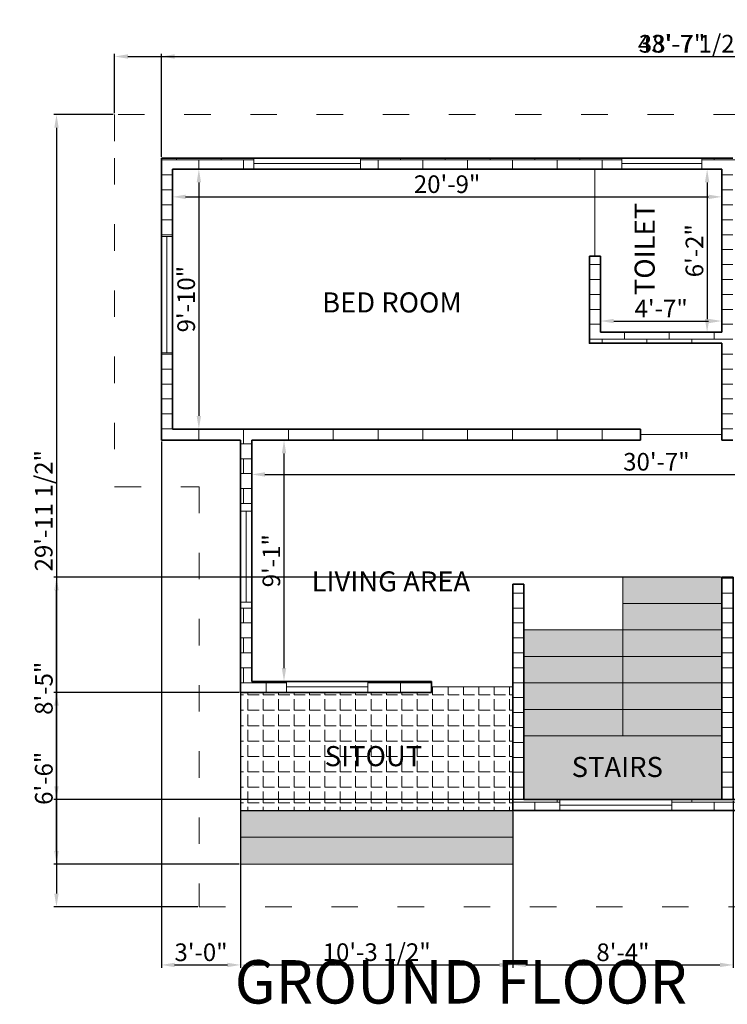
# Model space of a CAD drawing. Units: millimetres. Extents: x 1518 to 2850, y 936 to 2174.
# Tile 2 of 5: x 1686 to 2007, y 1697 to 2143. Entities that reach past the tile are written whole.
import ezdxf

# ---------------------------------------------------------------- set-up
doc = ezdxf.new("R2010")
doc.units = ezdxf.units.MM
doc.linetypes.add('ACAD_ISO03W100', pattern=[30, 12, -18])
for name, color, linetype, lineweight, true_color in [('A-ANNO-DIMS', 9, 'Continuous', 18, 0xafd9aa), ('A-ANNO-TEXT', 85, 'Continuous', 25, 0x58ba48), ('A-AREA-IDEN', 31, 'Continuous', 18, 0xfecc66), ('A-DOOR', 244, 'Continuous', 20, 0x991b1e), ('A-FLOR-PATT', 252, 'Continuous', 13, 0x939598), ('A-GLAZ', 141, 'Continuous', 18, 0xadddf7), ('A-ROOF-OVHD', 177, 'ACAD_ISO03W100', 18, 0x293189)]:
    doc.layers.add(name, color=color, linetype=linetype, lineweight=lineweight, true_color=true_color)
for name, color, linetype, lineweight in [('A-FLOR', 7, 'Continuous', 25), ('A-FLOR-STRS', 7, 'Continuous', 20), ('A-FLOR-STRS-PATT', 7, 'Continuous', 13), ('A-WALL', 7, 'Continuous', 35), ('A-WALL-PATT', 7, 'Continuous', 13)]:
    doc.layers.add(name, color=color, linetype=linetype, lineweight=lineweight)
doc.styles.get("Standard").update_dxf_attribs({"font": 'arial.ttf'})
doc.dimstyles.new('ISO-25', dxfattribs={"dimtxt": 8, "dimasz": 6, "dimexe": 1.25, "dimexo": 0.625, "dimtad": 1, "dimdec": 0, "dimlunit": 3, "dimtxsty": 'Standard', "dimcen": 2.5, "dimadec": 0, "dimazin": 0, "dimtfac": 1, "dimtdec": 0, "dimtmove": 0, "dimatfit": 3, "dimfxl": 1, "dimarcsym": 0})

# ---------------------------------------------------------------- blocks, each defined once
blk = doc.blocks.new('*D1')
at = {"layer": 'A-ANNO-DIMS', "color": 0, "lineweight": -2, "transparency": 16777216}
for p, q in [((1755, 2074.9), (1755, 2061.71)), ((2004.13, 2074.9), (2004.13, 2061.71)), ((1761, 2062.96), (1998.13, 2062.96))]:
    blk.add_line(p, q, dxfattribs=at)
at = {"layer": 'A-ANNO-DIMS', "color": 0, "transparency": 16777216}
for points in [[(1761, 2063.96), (1761, 2061.96), (1755, 2062.96)], [(1998.13, 2063.96), (1998.13, 2061.96), (2004.13, 2062.96)]]:
    blk.add_solid(points, dxfattribs=at)
at = {"layer": 'Defpoints', "color": 0, "transparency": 16777216}
for p in [(1755, 2075.52), (2004.13, 2075.52), (2004.13, 2062.96)]:
    blk.add_point(p, dxfattribs=at)
at = {"layer": 'A-ANNO-DIMS', "color": 0, "transparency": 16777216, "insert": (1879.56, 2067.67), "char_height": 8, "attachment_point": 5}
blk.add_mtext('20\'-9"', dxfattribs=at)
blk = doc.blocks.new('*D2')
at = {"layer": 'A-ANNO-DIMS', "color": 0, "lineweight": -2, "transparency": 16777216}
for p, q in [((1755.63, 2075.52), (1768.24, 2075.52)), ((1766.99, 2069.52), (1766.99, 1963.6)), ((1755.63, 1957.6), (1768.24, 1957.6))]:
    blk.add_line(p, q, dxfattribs=at)
at = {"layer": 'A-ANNO-DIMS', "color": 0, "transparency": 16777216}
for points in [[(1765.99, 2069.52), (1767.99, 2069.52), (1766.99, 2075.52)], [(1765.99, 1963.6), (1767.99, 1963.6), (1766.99, 1957.6)]]:
    blk.add_solid(points, dxfattribs=at)
at = {"layer": 'Defpoints', "color": 0, "transparency": 16777216}
for p in [(1755, 2075.52), (1755, 1957.6), (1766.99, 1957.6)]:
    blk.add_point(p, dxfattribs=at)
at = {"layer": 'A-ANNO-DIMS', "color": 0, "transparency": 16777216, "insert": (1762.28, 2016.56), "char_height": 8, "attachment_point": 5, "rotation": 90}
blk.add_mtext('9\'-10"', dxfattribs=at)
blk = doc.blocks.new('*D3')
at = {"layer": 'A-ANNO-DIMS', "color": 0, "lineweight": -2, "transparency": 16777216}
for p, q in [((1949.13, 2002.15), (1949.13, 2007.88)), ((1955.13, 2006.63), (1998.13, 2006.63)), ((2004.13, 2002.15), (2004.13, 2007.88))]:
    blk.add_line(p, q, dxfattribs=at)
at = {"layer": 'A-ANNO-DIMS', "color": 0, "transparency": 16777216}
for points in [[(1955.13, 2007.63), (1955.13, 2005.63), (1949.13, 2006.63)], [(1998.13, 2007.63), (1998.13, 2005.63), (2004.13, 2006.63)]]:
    blk.add_solid(points, dxfattribs=at)
at = {"layer": 'Defpoints', "color": 0, "transparency": 16777216}
for p in [(2004.13, 2006.63), (1949.13, 2001.52), (2004.13, 2001.52)]:
    blk.add_point(p, dxfattribs=at)
at = {"layer": 'A-ANNO-DIMS', "color": 0, "transparency": 16777216, "insert": (1976.63, 2011.25), "char_height": 8, "attachment_point": 5}
blk.add_mtext('4\'-7"', dxfattribs=at)
blk = doc.blocks.new('*D4')
at = {"layer": 'A-ANNO-DIMS', "color": 0, "lineweight": -2, "transparency": 16777216}
for p, q in [((2003.5, 2075.52), (1996.23, 2075.52)), ((1997.48, 2069.52), (1997.48, 2007.52)), ((2003.5, 2001.52), (1996.23, 2001.52))]:
    blk.add_line(p, q, dxfattribs=at)
at = {"layer": 'A-ANNO-DIMS', "color": 0, "transparency": 16777216}
for points in [[(1996.48, 2069.52), (1998.48, 2069.52), (1997.48, 2075.52)], [(1996.48, 2007.52), (1998.48, 2007.52), (1997.48, 2001.52)]]:
    blk.add_solid(points, dxfattribs=at)
at = {"layer": 'Defpoints', "color": 0, "transparency": 16777216}
for p in [(2004.13, 2075.52), (1997.48, 2001.52), (2004.13, 2001.52)]:
    blk.add_point(p, dxfattribs=at)
at = {"layer": 'A-ANNO-DIMS', "color": 0, "transparency": 16777216, "insert": (1992.77, 2038.52), "char_height": 8, "attachment_point": 5, "rotation": 90}
blk.add_mtext('6\'-2"', dxfattribs=at)
blk = doc.blocks.new('*D5')
at = {"layer": 'A-ANNO-DIMS', "color": 0, "lineweight": -2, "transparency": 16777216}
for p, q in [((1790.95, 1951.97), (1790.95, 1935.8)), ((2158.01, 1951.97), (2158.01, 1935.8)), ((1796.95, 1937.05), (2152.01, 1937.05))]:
    blk.add_line(p, q, dxfattribs=at)
at = {"layer": 'A-ANNO-DIMS', "color": 0, "transparency": 16777216}
for points in [[(1796.95, 1938.05), (1796.95, 1936.05), (1790.95, 1937.05)], [(2152.01, 1938.05), (2152.01, 1936.05), (2158.01, 1937.05)]]:
    blk.add_solid(points, dxfattribs=at)
at = {"layer": 'Defpoints', "color": 0, "transparency": 16777216}
for p in [(1790.95, 1952.6), (2158.01, 1952.6), (2158.01, 1937.05)]:
    blk.add_point(p, dxfattribs=at)
at = {"layer": 'A-ANNO-DIMS', "color": 0, "transparency": 16777216, "insert": (1974.48, 1941.76), "char_height": 8, "attachment_point": 5}
blk.add_mtext('30\'-7"', dxfattribs=at)
blk = doc.blocks.new('*D6')
at = {"layer": 'A-ANNO-DIMS', "color": 0, "lineweight": -2, "transparency": 16777216}
for p, q in [((1791.58, 1952.6), (1806.86, 1952.6)), ((1805.61, 1849.2), (1805.61, 1946.6)), ((1791.58, 1843.2), (1806.86, 1843.2))]:
    blk.add_line(p, q, dxfattribs=at)
at = {"layer": 'A-ANNO-DIMS', "color": 0, "transparency": 16777216}
for points in [[(1804.61, 1946.6), (1806.61, 1946.6), (1805.61, 1952.6)], [(1804.61, 1849.2), (1806.61, 1849.2), (1805.61, 1843.2)]]:
    blk.add_solid(points, dxfattribs=at)
at = {"layer": 'Defpoints', "color": 0, "transparency": 16777216}
for p in [(1790.95, 1952.6), (1805.61, 1952.6), (1790.95, 1843.2)]:
    blk.add_point(p, dxfattribs=at)
at = {"layer": 'A-ANNO-DIMS', "color": 0, "transparency": 16777216, "insert": (1800.9, 1897.9), "char_height": 8, "attachment_point": 5, "rotation": 90}
blk.add_mtext('9\'-1"', dxfattribs=at)
blk = doc.blocks.new('*D32')
at = {"layer": 'A-ANNO-DIMS', "color": 0, "lineweight": -2, "transparency": 16777216}
for p, q in [((1750, 2081.15), (1750, 2127.88)), ((1756, 2126.63), (2207.13, 2126.63)), ((2213.13, 2081.15), (2213.13, 2127.88))]:
    blk.add_line(p, q, dxfattribs=at)
at = {"layer": 'A-ANNO-DIMS', "color": 0, "transparency": 16777216}
for points in [[(1756, 2127.63), (1756, 2125.63), (1750, 2126.63)], [(2207.13, 2127.63), (2207.13, 2125.63), (2213.13, 2126.63)]]:
    blk.add_solid(points, dxfattribs=at)
at = {"layer": 'Defpoints', "color": 0, "transparency": 16777216}
for p in [(2213.13, 2126.63), (1750, 2080.52), (2213.13, 2080.52)]:
    blk.add_point(p, dxfattribs=at)
at = {"layer": 'A-ANNO-DIMS', "color": 0, "transparency": 16777216, "insert": (1981.56, 2131.34), "char_height": 8, "attachment_point": 5}
blk.add_mtext('38\'-7"', dxfattribs=at)
blk = doc.blocks.new('*D34')
at = {"layer": 'A-ANNO-DIMS', "color": 0, "lineweight": -2, "transparency": 16777216}
for p, q in [((1750, 1951.97), (1750, 1713.31)), ((1785.95, 1951.97), (1785.95, 1713.31)), ((1756, 1714.56), (1779.95, 1714.56))]:
    blk.add_line(p, q, dxfattribs=at)
at = {"layer": 'A-ANNO-DIMS', "color": 0, "transparency": 16777216}
for points in [[(1756, 1715.56), (1756, 1713.56), (1750, 1714.56)], [(1779.95, 1715.56), (1779.95, 1713.56), (1785.95, 1714.56)]]:
    blk.add_solid(points, dxfattribs=at)
at = {"layer": 'Defpoints', "color": 0, "transparency": 16777216}
for p in [(1750, 1952.6), (1785.95, 1952.6), (1785.95, 1714.56)]:
    blk.add_point(p, dxfattribs=at)
at = {"layer": 'A-ANNO-DIMS', "color": 0, "transparency": 16777216, "insert": (1767.98, 1719.27), "char_height": 8, "attachment_point": 5}
blk.add_mtext('3\'-0"', dxfattribs=at)
blk = doc.blocks.new('*D35')
at = {"layer": 'A-ANNO-DIMS', "color": 0, "lineweight": -2, "transparency": 16777216}
for p, q in [((1785.95, 1784), (1785.95, 1713.31)), ((1909.3, 1783.97), (1909.3, 1713.31)), ((1791.95, 1714.56), (1903.3, 1714.56))]:
    blk.add_line(p, q, dxfattribs=at)
at = {"layer": 'A-ANNO-DIMS', "color": 0, "transparency": 16777216}
for points in [[(1791.95, 1715.56), (1791.95, 1713.56), (1785.95, 1714.56)], [(1903.3, 1715.56), (1903.3, 1713.56), (1909.3, 1714.56)]]:
    blk.add_solid(points, dxfattribs=at)
at = {"layer": 'Defpoints', "color": 0, "transparency": 16777216}
for p in [(1785.95, 1784.62), (1909.3, 1784.6), (1909.3, 1714.56)]:
    blk.add_point(p, dxfattribs=at)
at = {"layer": 'A-ANNO-DIMS', "color": 0, "transparency": 16777216, "insert": (1847.63, 1719.32), "char_height": 8, "attachment_point": 5}
blk.add_mtext('10\'-3 1/2"', dxfattribs=at)
blk = doc.blocks.new('*D36')
at = {"layer": 'A-ANNO-DIMS', "color": 0, "lineweight": -2, "transparency": 16777216}
for p, q in [((2009.3, 1788.97), (2009.3, 1713.31)), ((1909.3, 1783.97), (1909.3, 1713.31)), ((1915.3, 1714.56), (2003.3, 1714.56))]:
    blk.add_line(p, q, dxfattribs=at)
at = {"layer": 'A-ANNO-DIMS', "color": 0, "transparency": 16777216}
for points in [[(1915.3, 1715.56), (1915.3, 1713.56), (1909.3, 1714.56)], [(2003.3, 1715.56), (2003.3, 1713.56), (2009.3, 1714.56)]]:
    blk.add_solid(points, dxfattribs=at)
at = {"layer": 'Defpoints', "color": 0, "transparency": 16777216}
for p in [(2009.3, 1789.6), (1909.3, 1784.6), (2009.3, 1714.56)]:
    blk.add_point(p, dxfattribs=at)
at = {"layer": 'A-ANNO-DIMS', "color": 0, "transparency": 16777216, "insert": (1959.3, 1719.27), "char_height": 8, "attachment_point": 5}
blk.add_mtext('8\'-4"', dxfattribs=at)
blk = doc.blocks.new('*D38')
at = {"layer": 'A-ANNO-DIMS', "color": 0, "lineweight": -2, "transparency": 16777216}
for p, q in [((2003.5, 1890.49), (1701.19, 1890.49)), ((1702.44, 1795.6), (1702.44, 1884.49)), ((2003.5, 1789.6), (1701.19, 1789.6))]:
    blk.add_line(p, q, dxfattribs=at)
at = {"layer": 'A-ANNO-DIMS', "color": 0, "transparency": 16777216}
for points in [[(1701.44, 1884.49), (1703.44, 1884.49), (1702.44, 1890.49)], [(1701.44, 1795.6), (1703.44, 1795.6), (1702.44, 1789.6)]]:
    blk.add_solid(points, dxfattribs=at)
at = {"layer": 'Defpoints', "color": 0, "transparency": 16777216}
for p in [(1702.44, 1890.49), (2004.13, 1890.49), (2004.13, 1789.6)]:
    blk.add_point(p, dxfattribs=at)
at = {"layer": 'A-ANNO-DIMS', "color": 0, "transparency": 16777216, "insert": (1697.74, 1840.05), "char_height": 8, "attachment_point": 5, "rotation": 90}
blk.add_mtext('8\'-5"', dxfattribs=at)
blk = doc.blocks.new('*D39')
at = {"layer": 'A-ANNO-DIMS', "color": 0, "lineweight": -2, "transparency": 16777216}
for p, q in [((1785.33, 1838.2), (1701.19, 1838.2)), ((1702.44, 1766.21), (1702.44, 1832.2)), ((1785.33, 1760.21), (1701.19, 1760.21))]:
    blk.add_line(p, q, dxfattribs=at)
at = {"layer": 'A-ANNO-DIMS', "color": 0, "transparency": 16777216}
for points in [[(1701.44, 1832.2), (1703.44, 1832.2), (1702.44, 1838.2)], [(1701.44, 1766.21), (1703.44, 1766.21), (1702.44, 1760.21)]]:
    blk.add_solid(points, dxfattribs=at)
at = {"layer": 'Defpoints', "color": 0, "transparency": 16777216}
for p in [(1702.44, 1838.2), (1785.95, 1838.2), (1785.95, 1760.21)]:
    blk.add_point(p, dxfattribs=at)
at = {"layer": 'A-ANNO-DIMS', "color": 0, "transparency": 16777216, "insert": (1697.74, 1799.21), "char_height": 8, "attachment_point": 5, "rotation": 90}
blk.add_mtext('6\'-6"', dxfattribs=at)
blk = doc.blocks.new('*D40')
at = {"layer": 'A-ANNO-DIMS', "color": 0, "lineweight": -2, "transparency": 16777216}
for p, q in [((1728.79, 2100.9), (1728.79, 2127.88)), ((1734.79, 2126.63), (2246.4, 2126.63)), ((2252.4, 2100.9), (2252.4, 2127.88))]:
    blk.add_line(p, q, dxfattribs=at)
at = {"layer": 'A-ANNO-DIMS', "color": 0, "transparency": 16777216}
for points in [[(1734.79, 2127.63), (1734.79, 2125.63), (1728.79, 2126.63)], [(2246.4, 2127.63), (2246.4, 2125.63), (2252.4, 2126.63)]]:
    blk.add_solid(points, dxfattribs=at)
at = {"layer": 'Defpoints', "color": 0, "transparency": 16777216}
for p in [(2252.4, 2126.63), (1728.79, 2100.28), (2252.4, 2100.28)]:
    blk.add_point(p, dxfattribs=at)
at = {"layer": 'A-ANNO-DIMS', "color": 0, "transparency": 16777216, "insert": (1990.6, 2131.39), "char_height": 8, "attachment_point": 5}
blk.add_mtext('43\'-7 1/2"', dxfattribs=at)
blk = doc.blocks.new('*D41')
at = {"layer": 'A-ANNO-DIMS', "color": 0, "lineweight": -2, "transparency": 16777216}
for p, q in [((1728.17, 2100.28), (1701.19, 2100.28)), ((1702.44, 2094.28), (1702.44, 1746.91)), ((1766.47, 1740.91), (1701.19, 1740.91))]:
    blk.add_line(p, q, dxfattribs=at)
at = {"layer": 'A-ANNO-DIMS', "color": 0, "transparency": 16777216}
for points in [[(1701.44, 2094.28), (1703.44, 2094.28), (1702.44, 2100.28)], [(1701.44, 1746.91), (1703.44, 1746.91), (1702.44, 1740.91)]]:
    blk.add_solid(points, dxfattribs=at)
at = {"layer": 'Defpoints', "color": 0, "transparency": 16777216}
for p in [(1728.79, 2100.28), (1702.44, 1740.91), (1767.1, 1740.91)]:
    blk.add_point(p, dxfattribs=at)
at = {"layer": 'A-ANNO-DIMS', "color": 0, "transparency": 16777216, "insert": (1697.68, 1920.59), "char_height": 8, "attachment_point": 5, "rotation": 90}
blk.add_mtext('29\'-11 1/2"', dxfattribs=at)

msp = doc.modelspace()

# ---------------------------------------------------------------- hatches: boundary and pattern name
at = {"layer": 'A-FLOR-PATT'}
h = msp.add_hatch(dxfattribs=at)
h.set_pattern_fill('ANGLE', color=256)
h.set_pattern_definition([(0, (-61.84, 0), (0, 6.985), [5.08, -1.905]), (90, (-61.84, 0), (-6.985, 4e-16), [5.08, -1.905])])
h.paths.add_polyline_path([(1909.3, 1784.6), (1909.3, 1838.2), (1909.3, 1840.7), (1872.42, 1840.7), (1872.42, 1838.2), (1785.95, 1838.2), (1785.95, 1784.62)])
h.paths.add_polyline_path([(2134.13, 2015.52), (2134.13, 1993.83), (2131.63, 1993.83), (2131.63, 1957.6), (2134.13, 1957.6), (2208.13, 1957.6), (2213.13, 1957.6), (2213.13, 1987.59), (2208.13, 1987.59), (2208.13, 2015.52)])
at = {"layer": 'A-FLOR-STRS-PATT'}
h = msp.add_hatch(dxfattribs=at)
h.set_pattern_fill('AR-RROOF', color=256, scale=0.1)
h.set_pattern_definition([(0, (-61.8398, 0), (5.588, 2.54), [38.1, -5.08, 12.7, -2.54]), (0, (-58.4616, 1.27), (-2.54, 3.3782), [7.62, -0.8382, 15.24, -1.905]), (0, (-60.5698, 2.159), (13.208, 1.7018), [20.32, -3.556, 10.16, -2.54])])
h.paths.add_polyline_path([(1909.3, 1784.6), (1785.95, 1784.62), (1785.95, 1772.51), (1909.3, 1772.51)])
h.paths.add_polyline_path([(1909.3, 1772.51), (1785.95, 1772.51), (1785.95, 1760.21), (1909.3, 1760.21)])
h.paths.add_polyline_path([(2004.13, 1830.49), (1959.21, 1830.49), (1959.21, 1818.49), (2004.13, 1818.49)])
h.paths.add_polyline_path([(2004.13, 1818.49), (1959.21, 1818.49), (1914.3, 1818.49), (1914.3, 1789.6), (2004.13, 1789.6)])
h.paths.add_polyline_path([(1959.21, 1830.49), (1914.3, 1830.49), (1914.3, 1818.49), (1959.21, 1818.49)])
h.paths.add_polyline_path([(1959.21, 1842.49), (1914.3, 1842.49), (1914.3, 1830.49), (1959.21, 1830.49)])
h.paths.add_polyline_path([(1959.21, 1854.49), (1914.3, 1854.49), (1914.3, 1842.49), (1959.21, 1842.49)])
h.paths.add_polyline_path([(1959.21, 1866.49), (1914.3, 1866.49), (1914.3, 1854.49), (1959.21, 1854.49)])
h.paths.add_polyline_path([(2004.13, 1890.49), (1959.21, 1890.49), (1959.21, 1878.49), (2004.13, 1878.49)])
h.paths.add_polyline_path([(2004.13, 1878.49), (1959.21, 1878.49), (1959.21, 1866.49), (2004.13, 1866.49)])
h.paths.add_polyline_path([(2004.13, 1866.49), (1959.21, 1866.49), (1959.21, 1854.49), (2004.13, 1854.49)])
h.paths.add_polyline_path([(2004.13, 1854.49), (1959.21, 1854.49), (1959.21, 1842.49), (2004.13, 1842.49)])
h.paths.add_polyline_path([(2004.13, 1842.49), (1959.21, 1842.49), (1959.21, 1830.49), (2004.13, 1830.49)])
h.paths.add_polyline_path([(2228.7, 1987.6), (2220.91, 1987.6), (2220.91, 1957.6), (2228.7, 1957.6)])
h.paths.add_polyline_path([(2220.91, 1987.6), (2213.13, 1987.6), (2213.13, 1957.6), (2220.91, 1957.6)])
h.paths.add_polyline_path([(2228.7, 2050.52), (2220.91, 2050.52), (2220.91, 2020.52), (2228.7, 2020.52)])
h.paths.add_polyline_path([(2220.91, 2050.52), (2213.13, 2050.52), (2213.13, 2020.52), (2220.91, 2020.52)])
at = {"layer": 'A-WALL-PATT'}
h = msp.add_hatch(dxfattribs=at)
h.set_pattern_fill('AR-BRSTD', color=256, scale=0.1)
h.set_pattern_definition([(0, (-61.84, 0), (0, 6.77418), []), (90, (-61.84, 0), (-10.16, 6.77418), [6.77418, -6.77418])])
h.paths.add_polyline_path([(1750, 1952.6), (1785.95, 1952.6), (1785.95, 1920.45), (1790.95, 1920.45), (1790.95, 1952.6), (1909.3, 1952.6), (1914.3, 1952.6), (1949.13, 1952.6), (1967.34, 1952.6), (1967.34, 1957.6), (1949.13, 1957.6), (1755, 1957.6), (1755, 1992.17), (1750, 1992.17)])
h.paths.add_polyline_path([(1791.93, 2075.52), (1791.93, 2080.52), (1750, 2080.52), (1750, 2045), (1755, 2045), (1755, 2075.52)])
h.paths.add_polyline_path([(1944.13, 2075.52), (1949.13, 2075.52), (1958.76, 2075.52), (1958.76, 2080.52), (1949.13, 2080.52), (1840.29, 2080.52), (1840.29, 2075.52)])
h.paths.add_polyline_path([(2004.13, 2075.52), (2004.13, 2001.52), (1949.13, 2001.52), (1949.13, 2036.02), (1944.13, 2036.02), (1944.13, 1996.52), (1949.13, 1996.52), (2004.13, 1996.52), (2004.13, 1957.6), (2004.13, 1952.6), (2009.13, 1952.6), (2009.13, 1957.6), (2009.13, 1996.52), (2009.13, 2075.52), (2036.64, 2075.52), (2036.64, 2080.52), (2009.13, 2080.52), (1995.08, 2080.52), (1995.08, 2075.52)])
h.paths.add_polyline_path([(2101.06, 2080.52), (2101.06, 2075.52), (2129.13, 2075.52), (2129.13, 1993.83), (2134.13, 1993.83), (2134.13, 2015.52), (2208.13, 2015.52), (2213.13, 2015.52), (2213.13, 2020.52), (2208.13, 2020.52), (2134.13, 2020.52), (2134.13, 2075.52), (2155.67, 2075.52), (2155.67, 2080.52), (2129.13, 2080.52)])
h.paths.add_polyline_path([(2180.68, 2080.52), (2180.68, 2075.52), (2208.13, 2075.52), (2208.13, 2050.52), (2213.13, 2050.52), (2213.13, 2080.52)], flags=17)
h.paths.add_polyline_path([(2129.13, 1952.6), (2158.01, 1952.6), (2158.01, 1918.63), (2163.01, 1918.63), (2163.01, 1952.6), (2213.13, 1952.6), (2213.13, 1957.6), (2208.13, 1957.6), (2134.13, 1957.6), (2129.13, 1957.6), (2045.26, 1957.6), (2045.26, 1952.6)])
h.paths.add_polyline_path([(2116.7, 1789.6), (2116.7, 1784.6), (2163.01, 1784.6), (2163.01, 1838.76), (2158.01, 1838.76), (2158.01, 1789.6)])
h.paths.add_polyline_path([(2047.7, 1784.6), (2047.7, 1789.6), (1981.4, 1789.6), (1981.4, 1784.6)])
h.paths.add_polyline_path([(2009.3, 1890.49), (2004.13, 1890.49), (2004.13, 1789.6), (2009.3, 1789.6)])
h.paths.add_polyline_path([(1930.65, 1784.6), (1930.65, 1789.6), (1914.3, 1789.6), (1914.3, 1887.35), (1909.3, 1887.35), (1909.3, 1843.2), (1909.3, 1838.2), (1909.3, 1784.6)])
h.paths.add_polyline_path([(1872.42, 1838.2), (1872.42, 1843.2), (1843.67, 1843.2), (1843.67, 1838.2)])
h.paths.add_polyline_path([(1790.95, 1843.2), (1790.95, 1879.12), (1785.95, 1879.12), (1785.95, 1838.2), (1806.76, 1838.2), (1806.76, 1843.2)])

# ---------------------------------------------------------------- linework, layer by layer
at = {"layer": 'A-DOOR'}
for p, q in [((1946.63, 2036.02), (1946.63, 2075.52)), ((1967.34, 1955.1), (2004.13, 1955.1)), ((1872.42, 1840.7), (1909.3, 1840.7))]:
    msp.add_line(p, q, dxfattribs=at)
at = {"layer": 'A-FLOR'}
for p, q in [((1785.95, 1838.2), (1785.95, 1784.62)), ((1785.95, 1784.62), (1909.3, 1784.6))]:
    msp.add_line(p, q, dxfattribs=at)
at = {"layer": 'A-FLOR-STRS'}
for p, q in [((1959.21, 1818.49), (1959.21, 1890.49)), ((1959.21, 1890.49), (2004.13, 1890.49)), ((2004.13, 1890.49), (2004.13, 1878.49)), ((2004.13, 1878.49), (1959.21, 1878.49)), ((1959.21, 1878.49), (1959.21, 1866.49)), ((1959.21, 1866.49), (1914.3, 1866.49)), ((1959.21, 1866.49), (2004.13, 1866.49)), ((2004.13, 1866.49), (2004.13, 1854.49)), ((1959.21, 1854.49), (1914.3, 1854.49)), ((2004.13, 1854.49), (1959.21, 1854.49)), ((1959.21, 1854.49), (1959.21, 1842.49)), ((1959.21, 1842.49), (1914.3, 1842.49)), ((1959.21, 1842.49), (2004.13, 1842.49)), ((2004.13, 1842.49), (2004.13, 1830.49)), ((1959.21, 1830.49), (1914.3, 1830.49)), ((2004.13, 1830.49), (1959.21, 1830.49)), ((1959.21, 1830.49), (1959.21, 1818.49)), ((1914.3, 1818.49), (2004.13, 1818.49)), ((1959.21, 1818.49), (2004.13, 1818.49)), ((1785.95, 1784.62), (1785.95, 1772.51)), ((1909.3, 1772.51), (1909.3, 1784.6)), ((1909.3, 1784.6), (1909.3, 1760.21)), ((1785.95, 1772.51), (1909.3, 1772.51)), ((1785.95, 1760.21), (1785.95, 1772.51)), ((1909.3, 1760.21), (1785.95, 1760.21))]:
    msp.add_line(p, q, dxfattribs=at)
at = {"layer": 'A-GLAZ'}
for p, q in [((1791.93, 2078.02), (1840.29, 2078.02)), ((1958.76, 2078.02), (1995.08, 2078.02)), ((1752.5, 1992.17), (1752.5, 2045)), ((1788.45, 1879.12), (1788.45, 1920.45)), ((1806.76, 1840.7), (1843.67, 1840.7)), ((1930.65, 1787.1), (1981.4, 1787.1))]:
    msp.add_line(p, q, dxfattribs=at)
for points in [[(1791.93, 2080.52), (1840.29, 2080.52), (1840.29, 2075.52), (1791.93, 2075.52)], [(1995.08, 2080.52), (1958.76, 2080.52), (1958.76, 2075.52), (1995.08, 2075.52)], [(1750, 2045), (1755, 2045), (1755, 1992.17), (1750, 1992.17)], [(1790.95, 1920.45), (1785.95, 1920.45), (1785.95, 1879.12), (1790.95, 1879.12)], [(1806.76, 1843.2), (1843.67, 1843.2), (1843.67, 1838.2), (1806.76, 1838.2)], [(1930.65, 1789.6), (1981.4, 1789.6), (1981.4, 1784.6), (1930.65, 1784.6)]]:
    msp.add_lwpolyline(points, close=True, dxfattribs=at)
at = {"layer": 'A-ROOF-OVHD'}
for p, q in [((2252.4, 2100.28), (1728.79, 2100.28)), ((1728.79, 2100.28), (1728.79, 2080.52)), ((1728.79, 2080.52), (1728.79, 1931.5)), ((1728.79, 1931.5), (1767.1, 1931.5)), ((1767.1, 1931.5), (1767.1, 1740.91)), ((1767.1, 1740.91), (2189.67, 1740.91))]:
    msp.add_line(p, q, dxfattribs=at)
at = {"layer": 'A-WALL'}
for p, q in [((1750, 2080.52), (1949.13, 2080.52)), ((1750, 1952.6), (1750, 2080.52)), ((1949.13, 2080.52), (2009.13, 2080.52)), ((1755, 2075.52), (1944.13, 2075.52)), ((1755, 1957.6), (1755, 2075.52)), ((1949.13, 2075.52), (2004.13, 2075.52)), ((2004.13, 2075.52), (2004.13, 2001.52)), ((1944.13, 2036.02), (1944.13, 1996.52)), ((1949.13, 2036.02), (1949.13, 2001.52)), ((2004.13, 2001.52), (1949.13, 2001.52)), ((2004.13, 1996.52), (1949.13, 1996.52)), ((2004.13, 1957.6), (2004.13, 1996.52)), ((1949.13, 1957.6), (1755, 1957.6)), ((1949.13, 1957.6), (1967.34, 1957.6)), ((1785.95, 1952.6), (1750, 1952.6)), ((1785.95, 1952.6), (1785.95, 1838.2)), ((1790.95, 1952.6), (1790.95, 1843.2)), ((1909.3, 1952.6), (1790.95, 1952.6)), ((1949.13, 1952.6), (1914.3, 1952.6)), ((1949.13, 1952.6), (1967.34, 1952.6)), ((2004.13, 1952.6), (2009.13, 1952.6)), ((1909.3, 1843.2), (1909.3, 1887.35)), ((1914.3, 1789.6), (1914.3, 1887.35)), ((1790.95, 1843.2), (1872.42, 1843.2)), ((1785.95, 1838.2), (1872.42, 1838.2)), ((1909.3, 1784.6), (1909.3, 1838.2)), ((2158.01, 1789.6), (1914.3, 1789.6)), ((2163.01, 1784.6), (1909.3, 1784.6))]:
    msp.add_line(p, q, dxfattribs=at)
for points in [[(1949.13, 2075.52), (1944.13, 2075.52)], [(1944.13, 2036.02), (1949.13, 2036.02)], [(1967.34, 1957.6), (1967.34, 1952.6)], [(2004.13, 1952.6), (2004.13, 1957.6)], [(1914.3, 1952.6), (1909.3, 1952.6)], [(2009.3, 1890.49), (2004.13, 1890.49)], [(2009.3, 1890.49), (2009.3, 1789.6), (2004.13, 1789.6), (2004.13, 1890.49)], [(1909.3, 1887.35), (1914.3, 1887.35)], [(1872.42, 1843.2), (1872.42, 1838.2)], [(1909.3, 1838.2), (1909.3, 1843.2)]]:
    msp.add_lwpolyline(points, dxfattribs=at)
msp.add_lwpolyline([(1949.13, 1996.52), (1944.13, 1996.52), (1944.13, 1996.52), (1949.13, 1996.52)], close=True, dxfattribs=at)

# ---------------------------------------------------------------- texts
at = {"layer": 'A-ANNO-TEXT'}
msp.add_text('GROUND FLOOR', height=19.6883, dxfattribs=at).set_placement((1783.27, 1697.05))
at = {"layer": 'A-AREA-IDEN'}
msp.add_text('TOILET', height=9.117, rotation=90, dxfattribs=at).set_placement((1973.72, 2018.37))
for s, height, p in [('BED ROOM', 9.117, (1822.88, 2010.51)), ('LIVING AREA', 9.1171, (1818.11, 1883.96)), ('SITOUT', 9.117, (1824.08, 1804.71)), ('STAIRS', 9.117, (1936.05, 1799.8))]:
    msp.add_text(s, height=height, dxfattribs=at).set_placement(p)

# ---------------------------------------------------------------- dimensions: what is measured, and where the dimension line sits
at = {"layer": 'A-ANNO-DIMS'}
for base, p1, p2, override, picture, middle in [((2252.4, 2126.63), (1728.79, 2100.28), (2252.4, 2100.28), {"dimdec": 1, "dimlfac": 1, "dimrnd": 0, "dimzin": 1, "dimdsep": 46, "dimlunit": 4, "dimfrac": 2}, '*D40', (1990.6, 2131.39)), ((2213.13, 2126.63), (1750, 2080.52), (2213.13, 2080.52), {"dimdec": 1, "dimlfac": 1, "dimrnd": 0, "dimzin": 1, "dimdsep": 46, "dimlunit": 4, "dimfrac": 2}, '*D32', (1981.56, 2131.34)), ((2004.13, 2062.96), (1755, 2075.52), (2004.13, 2075.52), {"dimclrd": 0, "dimclre": 0, "dimclrt": 0}, '*D1', (1879.56, 2067.67)), ((2004.13, 2006.63), (1949.13, 2001.52), (2004.13, 2001.52), {"dimclrd": 0, "dimclre": 0, "dimclrt": 0}, '*D3', (1976.63, 2011.25)), ((1785.9546, 1714.5569), (1750.0017, 1952.5976), (1785.9546, 1952.5976), {"dimdec": 1, "dimlfac": 1, "dimrnd": 0, "dimzin": 1, "dimdsep": 46, "dimlunit": 4, "dimfrac": 2}, '*D34', (1767.9781, 1719.2693)), ((2158.01, 1937.05), (1790.95, 1952.6), (2158.01, 1952.6), {"dimclrd": 0, "dimclre": 0, "dimclrt": 0}, '*D5', (1974.48, 1941.76)), ((2009.3, 1714.56), (1909.3, 1784.6), (2009.3, 1789.6), {"dimdec": 1, "dimlfac": 1, "dimrnd": 0, "dimzin": 1, "dimdsep": 46, "dimlunit": 4, "dimfrac": 2}, '*D36', (1959.3, 1719.27)), ((1909.2979, 1714.5569), (1785.9546, 1784.6239), (1909.2979, 1784.5976), {"dimdec": 1, "dimlfac": 1, "dimrnd": 0, "dimzin": 1, "dimdsep": 46, "dimlunit": 4, "dimfrac": 2}, '*D35', (1847.6262, 1719.3211))]:
    dim = msp.add_linear_dim(base=base, p1=p1, p2=p2, dimstyle='ISO-25', override=override, dxfattribs=at)
    dim.commit()
    dim.dimension.update_dxf_attribs({"geometry": picture, "text_midpoint": middle})
for base, p1, p2, override, picture, middle in [((1702.44, 1740.91), (1728.79, 2100.28), (1767.1, 1740.91), {"dimdec": 1, "dimlfac": 1, "dimrnd": 0, "dimzin": 1, "dimdsep": 46, "dimlunit": 4, "dimfrac": 2}, '*D41', (1697.68, 1920.59)), ((1766.99, 1957.6), (1755, 2075.52), (1755, 1957.6), {"dimclrd": 0, "dimclre": 0, "dimclrt": 0}, '*D2', (1762.28, 2016.56)), ((1997.48, 2001.52), (2004.13, 2075.52), (2004.13, 2001.52), {"dimclrd": 0, "dimclre": 0, "dimclrt": 0}, '*D4', (1992.77, 2038.52)), ((1805.61, 1952.6), (1790.95, 1843.2), (1790.95, 1952.6), {"dimclrd": 0, "dimclre": 0, "dimclrt": 0}, '*D6', (1800.9, 1897.9)), ((1702.44, 1890.49), (2004.13, 1789.6), (2004.13, 1890.49), {"dimdec": 1, "dimlfac": 1, "dimrnd": 0, "dimzin": 1, "dimdsep": 46, "dimlunit": 4, "dimfrac": 2}, '*D38', (1697.74, 1840.05)), ((1702.44, 1838.2), (1785.95, 1760.21), (1785.95, 1838.2), {"dimdec": 1, "dimlfac": 1, "dimrnd": 0, "dimzin": 1, "dimdsep": 46, "dimlunit": 4, "dimfrac": 2}, '*D39', (1697.74, 1799.21))]:
    dim = msp.add_linear_dim(base=base, p1=p1, p2=p2, angle=90, dimstyle='ISO-25', override=override, dxfattribs=at)
    dim.commit()
    dim.dimension.update_dxf_attribs({"geometry": picture, "text_midpoint": middle})

doc.saveas('drawing.dxf')
